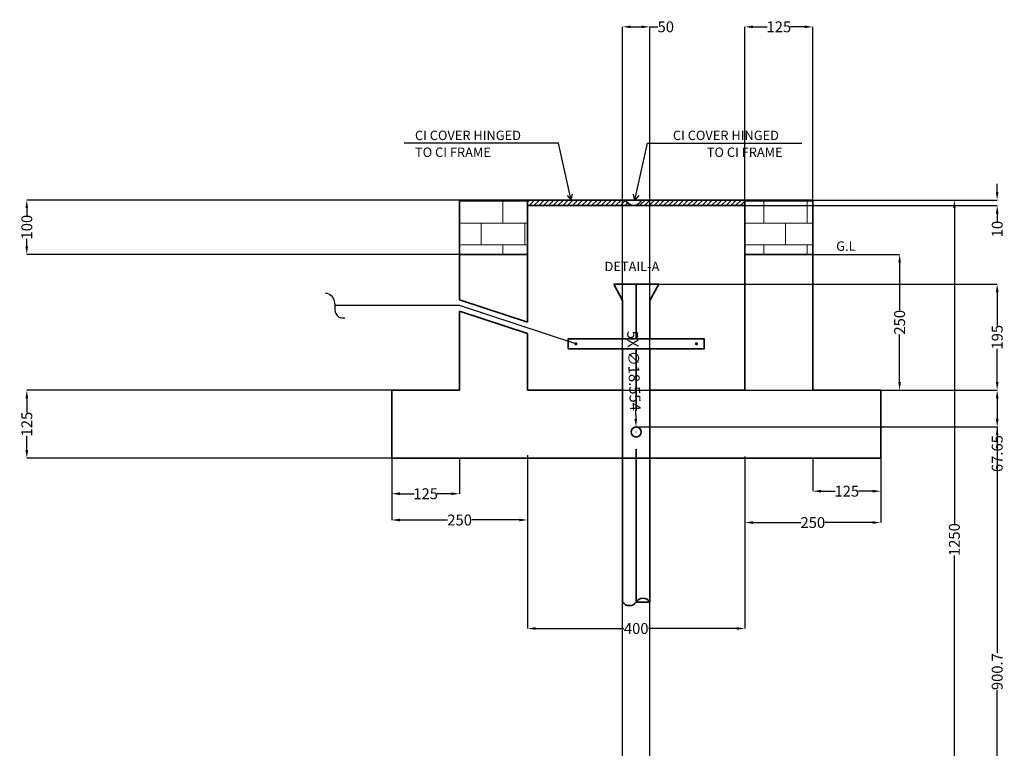
# Model space of a CAD drawing. Units: inches. Extents: x -129 to 2013, y -3652 to 814.
# Tile 5 of 5: x -129 to 1683, y -527 to 814. Entities that reach past the tile are written whole.
import ezdxf

# ---------------------------------------------------------------- set-up
doc = ezdxf.new("R2010")
doc.units = ezdxf.units.IN
doc.header["$MEASUREMENT"] = 0
for name, color, linetype, lineweight in [('A-ANNO-DIMS', 2, 'Continuous', 18), ('A-ANNO-TEXT', 7, 'Continuous', 25), ('A-DETL', 7, 'Continuous', 35), ('A-DETL-PATT', 8, 'Continuous', 13), ('E-GRND', 1, 'Continuous', 35)]:
    doc.layers.add(name, color=color, linetype=linetype, lineweight=lineweight)
doc.styles.get("Standard").update_dxf_attribs({"font": 'arial.ttf'})
doc.dimstyles.get("Standard").update_dxf_attribs({"dimtxt": 20, "dimasz": 15, "dimexe": 0.18, "dimexo": 0.0625, "dimgap": 0.09, "dimtad": 0, "dimdec": 0, "dimzin": 0, "dimdsep": 46, "dimtxsty": 'Standard', "dimcen": 0.09, "dimadec": 0, "dimazin": 0, "dimtfac": 1, "dimtdec": 0, "dimtofl": 0, "dimtmove": 0, "dimatfit": 3, "dimfxl": 1, "dimtolj": 1, "dimtzin": 0, "dimarcsym": 0})

# ---------------------------------------------------------------- blocks, each defined once
blk = doc.blocks.new('*D1')
at = {"layer": 'A-ANNO-DIMS', "color": 0, "lineweight": -2, "transparency": 16777216}
for p, q in [((1330.4, 382.4), (1490.1, 382.4)), ((1490, 367.4), (1490, 279.7)), ((1490, 147.4), (1490, 235)), ((1455.4, 132.4), (1490.1, 132.4))]:
    blk.add_line(p, q, dxfattribs=at)
at = {"layer": 'A-ANNO-DIMS', "color": 0, "transparency": 16777216}
for points in [[(1487.5, 367.4), (1492.5, 367.4), (1490, 382.4)], [(1487.5, 147.4), (1492.5, 147.4), (1490, 132.4)]]:
    blk.add_solid(points, dxfattribs=at)
at = {"layer": 'Defpoints', "color": 0, "transparency": 16777216}
for p in [(1330.3, 382.4), (1490, 382.4), (1455.3, 132.4)]:
    blk.add_point(p, dxfattribs=at)
at = {"layer": 'A-ANNO-DIMS', "color": 0, "transparency": 16777216, "insert": (1490, 257.4), "char_height": 20, "attachment_point": 5, "rotation": 90}
blk.add_mtext('\\A1;250', dxfattribs=at)
blk = doc.blocks.new('*D2')
at = {"layer": 'A-ANNO-DIMS', "color": 0, "lineweight": -2, "transparency": 16777216}
for p, q in [((1330.4, 482.4), (1591, 482.4)), ((1590.8, 467.4), (1590.8, -113.7)), ((1590.8, -752.6), (1590.8, -171.6)), ((1205.4, -767.6), (1591, -767.6))]:
    blk.add_line(p, q, dxfattribs=at)
at = {"layer": 'A-ANNO-DIMS', "color": 0, "transparency": 16777216}
for points in [[(1588.3, 467.4), (1593.3, 467.4), (1590.8, 482.4)], [(1588.3, -752.6), (1593.3, -752.6), (1590.8, -767.6)]]:
    blk.add_solid(points, dxfattribs=at)
at = {"layer": 'Defpoints', "color": 0, "transparency": 16777216}
for p in [(1330.3, 482.4), (1205.3, -767.6), (1590.8, -767.6)]:
    blk.add_point(p, dxfattribs=at)
at = {"layer": 'A-ANNO-DIMS', "color": 0, "transparency": 16777216, "insert": (1590.8, -142.6), "char_height": 20, "attachment_point": 5, "rotation": 90}
blk.add_mtext('\\A1;1250', dxfattribs=at)
blk = doc.blocks.new('*D4')
at = {"layer": 'A-ANNO-DIMS', "color": 0, "lineweight": -2, "transparency": 16777216}
for p, q in [((555.3, 7.3), (555.3, -58.3)), ((680.3, 7.3), (680.3, -58.3)), ((570.3, -58.2), (596.5, -58.2)), ((665.3, -58.2), (639.1, -58.2))]:
    blk.add_line(p, q, dxfattribs=at)
at = {"layer": 'A-ANNO-DIMS', "color": 0, "transparency": 16777216}
for points in [[(570.3, -55.7), (570.3, -60.7), (555.3, -58.2)], [(665.3, -55.7), (665.3, -60.7), (680.3, -58.2)]]:
    blk.add_solid(points, dxfattribs=at)
at = {"layer": 'Defpoints', "color": 0, "transparency": 16777216}
for p in [(555.3, 7.4), (680.3, 7.4), (680.3, -58.2)]:
    blk.add_point(p, dxfattribs=at)
at = {"layer": 'A-ANNO-DIMS', "color": 0, "transparency": 16777216, "insert": (617.8, -58.2), "char_height": 20, "attachment_point": 5}
blk.add_mtext('\\A1;125', dxfattribs=at)
blk = doc.blocks.new('*D5')
at = {"layer": 'A-ANNO-DIMS', "color": 0, "lineweight": -2, "transparency": 16777216}
for p, q in [((555.3, 7.3), (555.3, -106.7)), ((805.3, 12.7), (805.3, -106.7)), ((570.3, -106.5), (658, -106.5)), ((790.3, -106.5), (702.7, -106.5))]:
    blk.add_line(p, q, dxfattribs=at)
at = {"layer": 'A-ANNO-DIMS', "color": 0, "transparency": 16777216}
for points in [[(570.3, -104), (570.3, -109), (555.3, -106.5)], [(790.3, -104), (790.3, -109), (805.3, -106.5)]]:
    blk.add_solid(points, dxfattribs=at)
at = {"layer": 'Defpoints', "color": 0, "transparency": 16777216}
for p in [(555.3, 7.4), (805.3, 12.8), (805.3, -106.5)]:
    blk.add_point(p, dxfattribs=at)
at = {"layer": 'A-ANNO-DIMS', "color": 0, "transparency": 16777216, "insert": (680.3, -106.5), "char_height": 20, "attachment_point": 5}
blk.add_mtext('\\A1;250', dxfattribs=at)
blk = doc.blocks.new('*D6')
at = {"layer": 'A-ANNO-DIMS', "color": 0, "lineweight": -2, "transparency": 16777216}
for p, q in [((1330.3, 7.3), (1330.3, -53.6)), ((1455.3, 7.3), (1455.3, -53.6)), ((1345.3, -53.5), (1371.5, -53.5)), ((1440.3, -53.5), (1414.1, -53.5))]:
    blk.add_line(p, q, dxfattribs=at)
at = {"layer": 'A-ANNO-DIMS', "color": 0, "transparency": 16777216}
for points in [[(1345.3, -51), (1345.3, -56), (1330.3, -53.5)], [(1440.3, -51), (1440.3, -56), (1455.3, -53.5)]]:
    blk.add_solid(points, dxfattribs=at)
at = {"layer": 'Defpoints', "color": 0, "transparency": 16777216}
for p in [(1330.3, 7.4), (1455.3, 7.4), (1330.3, -53.5)]:
    blk.add_point(p, dxfattribs=at)
at = {"layer": 'A-ANNO-DIMS', "color": 0, "transparency": 16777216, "insert": (1392.8, -53.5), "char_height": 20, "attachment_point": 5}
blk.add_mtext('\\A1;125', dxfattribs=at)
blk = doc.blocks.new('*D7')
at = {"layer": 'A-ANNO-DIMS', "color": 0, "lineweight": -2, "transparency": 16777216}
for p, q in [((1455.3, 132.3), (1455.3, -111.4)), ((1205.3, 10.4), (1205.3, -111.4)), ((1220.3, -111.2), (1308, -111.2)), ((1440.3, -111.2), (1352.7, -111.2))]:
    blk.add_line(p, q, dxfattribs=at)
at = {"layer": 'A-ANNO-DIMS', "color": 0, "transparency": 16777216}
for points in [[(1220.3, -108.7), (1220.3, -113.7), (1205.3, -111.2)], [(1440.3, -108.7), (1440.3, -113.7), (1455.3, -111.2)]]:
    blk.add_solid(points, dxfattribs=at)
at = {"layer": 'Defpoints', "color": 0, "transparency": 16777216}
for p in [(1455.3, 132.4), (1205.3, 10.5), (1205.3, -111.2)]:
    blk.add_point(p, dxfattribs=at)
at = {"layer": 'A-ANNO-DIMS', "color": 0, "transparency": 16777216, "insert": (1330.3, -111.2), "char_height": 20, "attachment_point": 5}
blk.add_mtext('\\A1;250', dxfattribs=at)
blk = doc.blocks.new('*D8')
at = {"layer": 'A-ANNO-DIMS', "color": 0, "lineweight": -2, "transparency": 16777216}
for p, q in [((805.3, 7.3), (805.3, -306.4)), ((1205.3, 10.4), (1205.3, -306.4)), ((820.3, -306.2), (982.8, -306.2)), ((1190.3, -306.2), (1027.9, -306.2))]:
    blk.add_line(p, q, dxfattribs=at)
at = {"layer": 'A-ANNO-DIMS', "color": 0, "transparency": 16777216}
for points in [[(820.3, -303.7), (820.3, -308.7), (805.3, -306.2)], [(1190.3, -303.7), (1190.3, -308.7), (1205.3, -306.2)]]:
    blk.add_solid(points, dxfattribs=at)
at = {"layer": 'Defpoints', "color": 0, "transparency": 16777216}
for p in [(805.3, 7.4), (1205.3, 10.5), (805.3, -306.2)]:
    blk.add_point(p, dxfattribs=at)
at = {"layer": 'A-ANNO-DIMS', "color": 0, "transparency": 16777216, "insert": (1005.3, -306.2), "char_height": 20, "attachment_point": 5}
blk.add_mtext('\\A1;400', dxfattribs=at)
blk = doc.blocks.new('*D22')
at = {"layer": 'A-ANNO-DIMS', "color": 0, "lineweight": -2, "transparency": 16777216}
for p, q in [((555.3, 132.4), (-116.3, 132.4)), ((-116.2, 117.4), (-116.2, 91.2)), ((-116.2, 22.4), (-116.2, 48.5)), ((555.3, 7.4), (-116.3, 7.4))]:
    blk.add_line(p, q, dxfattribs=at)
at = {"layer": 'A-ANNO-DIMS', "color": 0, "transparency": 16777216}
for points in [[(-118.7, 117.4), (-113.7, 117.4), (-116.2, 132.4)], [(-118.7, 22.4), (-113.7, 22.4), (-116.2, 7.4)]]:
    blk.add_solid(points, dxfattribs=at)
at = {"layer": 'Defpoints', "color": 0, "transparency": 16777216}
for p in [(-116.2, 132.4), (555.3, 132.4), (555.3, 7.4)]:
    blk.add_point(p, dxfattribs=at)
at = {"layer": 'A-ANNO-DIMS', "color": 0, "transparency": 16777216, "insert": (-116.2, 69.9), "char_height": 20, "attachment_point": 5, "rotation": 90}
blk.add_mtext('\\A1;125', dxfattribs=at)
blk = doc.blocks.new('*D23')
at = {"layer": 'A-ANNO-DIMS', "color": 0, "lineweight": -2, "transparency": 16777216}
for p, q in [((680.3, 482.4), (-116.3, 482.4)), ((-116.2, 467.4), (-116.2, 453.6)), ((-116.2, 397.4), (-116.2, 411.2)), ((680.3, 382.4), (-116.3, 382.4))]:
    blk.add_line(p, q, dxfattribs=at)
at = {"layer": 'A-ANNO-DIMS', "color": 0, "transparency": 16777216}
for points in [[(-118.7, 467.4), (-113.7, 467.4), (-116.2, 482.4)], [(-118.7, 397.4), (-113.7, 397.4), (-116.2, 382.4)]]:
    blk.add_solid(points, dxfattribs=at)
at = {"layer": 'Defpoints', "color": 0, "transparency": 16777216}
for p in [(-116.2, 482.4), (680.3, 482.4), (680.3, 382.4)]:
    blk.add_point(p, dxfattribs=at)
at = {"layer": 'A-ANNO-DIMS', "color": 0, "transparency": 16777216, "insert": (-116.2, 432.4), "char_height": 20, "attachment_point": 5, "rotation": 90}
blk.add_mtext('\\A1;100', dxfattribs=at)
blk = doc.blocks.new('*D24')
at = {"layer": 'A-ANNO-DIMS', "color": 0, "lineweight": -2, "transparency": 16777216}
for p, q in [((1205.3, 482.4), (1205.3, 801.3)), ((1220.3, 801.1), (1246.5, 801.1)), ((1315.3, 801.1), (1289.1, 801.1)), ((1330.3, 482.4), (1330.3, 801.3))]:
    blk.add_line(p, q, dxfattribs=at)
at = {"layer": 'A-ANNO-DIMS', "color": 0, "transparency": 16777216}
for points in [[(1220.3, 803.6), (1220.3, 798.6), (1205.3, 801.1)], [(1315.3, 803.6), (1315.3, 798.6), (1330.3, 801.1)]]:
    blk.add_solid(points, dxfattribs=at)
at = {"layer": 'Defpoints', "color": 0, "transparency": 16777216}
for p in [(1330.3, 801.1), (1205.3, 482.4), (1330.3, 482.4)]:
    blk.add_point(p, dxfattribs=at)
at = {"layer": 'A-ANNO-DIMS', "color": 0, "transparency": 16777216, "insert": (1267.8, 801.1), "char_height": 20, "attachment_point": 5}
blk.add_mtext('\\A1;125', dxfattribs=at)
blk = doc.blocks.new('*D25')
at = {"layer": 'A-ANNO-DIMS', "color": 0, "lineweight": -2, "transparency": 16777216}
for p, q in [((1669.6, 497.4), (1669.6, 512.4)), ((805.4, 482.4), (1669.8, 482.4)), ((805.4, 472.4), (1669.8, 472.4)), ((1669.6, 457.4), (1669.6, 442.4))]:
    blk.add_line(p, q, dxfattribs=at)
at = {"layer": 'A-ANNO-DIMS', "color": 0, "transparency": 16777216}
for points in [[(1667.1, 497.4), (1672.1, 497.4), (1669.6, 482.4)], [(1667.1, 457.4), (1672.1, 457.4), (1669.6, 472.4)]]:
    blk.add_solid(points, dxfattribs=at)
at = {"layer": 'Defpoints', "color": 0, "transparency": 16777216}
for p in [(805.3, 482.4), (805.3, 472.4), (1669.6, 472.4)]:
    blk.add_point(p, dxfattribs=at)
at = {"layer": 'A-ANNO-DIMS', "color": 0, "transparency": 16777216, "insert": (1669.6, 428.9), "char_height": 20, "attachment_point": 5, "rotation": 90}
blk.add_mtext('\\A1;10', dxfattribs=at)
blk = doc.blocks.new('*D26')
at = {"layer": 'A-ANNO-DIMS', "color": 0, "lineweight": -2, "transparency": 16777216}
for p, q in [((980.3, -1867.6), (980.3, 801.3)), ((995.3, 801.1), (1015.3, 801.1)), ((1030.3, -1867.6), (1030.3, 801.3)), ((1030.3, 801.1), (1045.3, 801.1))]:
    blk.add_line(p, q, dxfattribs=at)
at = {"layer": 'A-ANNO-DIMS', "color": 0, "transparency": 16777216}
for points in [[(995.3, 803.6), (995.3, 798.6), (980.3, 801.1)], [(1015.3, 803.6), (1015.3, 798.6), (1030.3, 801.1)]]:
    blk.add_solid(points, dxfattribs=at)
at = {"layer": 'Defpoints', "color": 0, "transparency": 16777216}
for p in [(1030.3, 801.1), (980.3, -1867.6), (1030.3, -1867.6)]:
    blk.add_point(p, dxfattribs=at)
at = {"layer": 'A-ANNO-DIMS', "color": 0, "transparency": 16777216, "insert": (1059.7, 801.1), "char_height": 20, "attachment_point": 5}
blk.add_mtext('\\A1;50', dxfattribs=at)
blk = doc.blocks.new('*D27')
at = {"layer": 'A-ANNO-DIMS', "color": 0, "lineweight": -2, "transparency": 16777216}
for p, q in [((1046.7, 327.4), (1669.8, 327.4)), ((1669.6, 312.4), (1669.6, 251.2)), ((1669.6, 147.4), (1669.6, 208.5)), ((1205.4, 132.4), (1669.8, 132.4))]:
    blk.add_line(p, q, dxfattribs=at)
at = {"layer": 'A-ANNO-DIMS', "color": 0, "transparency": 16777216}
for points in [[(1667.1, 312.4), (1672.1, 312.4), (1669.6, 327.4)], [(1667.1, 147.4), (1672.1, 147.4), (1669.6, 132.4)]]:
    blk.add_solid(points, dxfattribs=at)
at = {"layer": 'Defpoints', "color": 0, "transparency": 16777216}
for p in [(1046.7, 327.4), (1205.3, 132.4), (1669.6, 132.4)]:
    blk.add_point(p, dxfattribs=at)
at = {"layer": 'A-ANNO-DIMS', "color": 0, "transparency": 16777216, "insert": (1669.6, 229.9), "char_height": 20, "attachment_point": 5, "rotation": 90}
blk.add_mtext('\\A1;195', dxfattribs=at)
blk = doc.blocks.new('*D28')
at = {"layer": 'A-ANNO-DIMS', "color": 0, "lineweight": -2, "transparency": 16777216}
for p, q in [((980.4, 132.4), (1669.8, 132.4)), ((1669.6, 117.4), (1669.6, 79.7)), ((1005.4, 64.7), (1669.8, 64.7)), ((1669.6, 64.7), (1669.6, 49.7))]:
    blk.add_line(p, q, dxfattribs=at)
at = {"layer": 'A-ANNO-DIMS', "color": 0, "transparency": 16777216}
for points in [[(1667.1, 117.4), (1672.1, 117.4), (1669.6, 132.4)], [(1667.1, 79.7), (1672.1, 79.7), (1669.6, 64.7)]]:
    blk.add_solid(points, dxfattribs=at)
at = {"layer": 'Defpoints', "color": 0, "transparency": 16777216}
for p in [(980.3, 132.4), (1005.3, 64.7), (1669.6, 64.7)]:
    blk.add_point(p, dxfattribs=at)
at = {"layer": 'A-ANNO-DIMS', "color": 0, "transparency": 16777216, "insert": (1669.6, 15.7), "char_height": 20, "attachment_point": 5, "rotation": 90}
blk.add_mtext('\\A1;67.65', dxfattribs=at)
blk = doc.blocks.new('*D29')
at = {"layer": 'A-ANNO-DIMS', "color": 0, "lineweight": -2, "transparency": 16777216}
for p, q in [((1005.4, 64.7), (1669.8, 64.7)), ((1669.6, 49.7), (1669.6, -351.8)), ((1669.6, -821), (1669.6, -419.5)), ((1005.4, -836), (1669.8, -836))]:
    blk.add_line(p, q, dxfattribs=at)
at = {"layer": 'A-ANNO-DIMS', "color": 0, "transparency": 16777216}
for points in [[(1667.1, 49.7), (1672.1, 49.7), (1669.6, 64.7)], [(1667.1, -821), (1672.1, -821), (1669.6, -836)]]:
    blk.add_solid(points, dxfattribs=at)
at = {"layer": 'Defpoints', "color": 0, "transparency": 16777216}
for p in [(1005.3, 64.7), (1005.3, -836), (1669.6, -836)]:
    blk.add_point(p, dxfattribs=at)
at = {"layer": 'A-ANNO-DIMS', "color": 0, "transparency": 16777216, "insert": (1669.6, -385.6), "char_height": 20, "attachment_point": 5, "rotation": 90}
blk.add_mtext('\\A1;900.7', dxfattribs=at)
blk = doc.blocks.new('*D34')
at = {"layer": 'A-ANNO-DIMS', "color": 0, "lineweight": -2, "transparency": 16777216}
for p, q in [((1003.9, 94.7), (1004.4, 79.7)), ((1005.2, 55.4), (1005.4, 55.4)), ((1005.3, 55.3), (1005.3, 55.5))]:
    blk.add_line(p, q, dxfattribs=at)
at = {"layer": 'A-ANNO-DIMS', "color": 0, "transparency": 16777216}
blk.add_solid([(1006.9, 79.8), (1001.9, 79.6), (1005, 64.7)], dxfattribs=at)
at = {"layer": 'Defpoints', "color": 0, "transparency": 16777216}
for p in [(1005, 64.7), (1005.7, 46.2)]:
    blk.add_point(p, dxfattribs=at)
at = {"layer": 'A-ANNO-DIMS', "color": 0, "transparency": 16777216, "insert": (1001.2, 168), "char_height": 20, "attachment_point": 5, "rotation": 272.0841}
blk.add_mtext('\\A1;5X ∅18.554', dxfattribs=at)

msp = doc.modelspace()

# ---------------------------------------------------------------- hatches: boundary and pattern name
at = {"layer": 'A-DETL-PATT'}
h = msp.add_hatch(dxfattribs=at)
h.set_pattern_fill('AR-B816', color=256, scale=5)
h.paths.add_polyline_path([(805.3299, 482.3603), (680.3299, 482.3603), (680.3299, 382.3603), (805.3299, 382.3603)])
h.paths.add_polyline_path([(1330.3299, 482.3603), (1205.3299, 482.3603), (1205.3299, 382.3603), (1330.3299, 382.3603)])
h = msp.add_hatch(dxfattribs=at)
h.set_pattern_fill('ANSI31', color=256, scale=50)
h.paths.add_polyline_path([(985.6513, 482.3603), (805.3299, 482.3603), (805.3299, 472.3603), (999.6786, 472.3603, -0.293221438)])
h.paths.add_polyline_path([(1205.3299, 482.3603), (1015.2644, 482.3603, -0.293221438), (1001.2372, 472.3603), (1205.3299, 472.3603)])

# ---------------------------------------------------------------- linework, layer by layer
at = {"layer": 'A-ANNO-TEXT'}
for points in [[(885.4212, 482.3603), (862.3427, 586.8686), (578.5573, 586.8686)], [(1002.9842, 482.3603), (1026.0627, 586.8686), (1309.8482, 586.8686)], [(878.2422, 490.9289), (885.4212, 482.3603), (888.3242, 493.1553)], [(1010.1632, 490.9289), (1002.9842, 482.3603), (1000.0813, 493.1553)], [(894.3429, 217.8056), (680.3299, 288.2653), (450.6375, 288.2653)]]:
    msp.add_lwpolyline(points, dxfattribs=at)
msp.add_open_spline([(433.1167, 311.7522), (437.1039, 310.5265), (447.7143, 307.2646), (451.4749, 289.5005), (450.2729, 275.0479), (458.3312, 265.1335), (465.1078, 265.27), (468.8937, 265.3463)], degree=3, knots=[0, 0, 0, 0, 11.88575847, 31.629827154, 46.748444814, 55.2513882, 66.015071682, 66.015071682, 66.015071682, 66.015071682], dxfattribs=at)
at = {"layer": 'A-DETL'}
for p, q in [((680.3299, 482.3603), (805.3299, 482.3603)), ((680.3299, 298.7933), (680.3299, 482.3603)), ((805.3299, 482.3603), (805.3299, 257.6395)), ((1330.3299, 482.3603), (805.3299, 482.3603)), ((805.3299, 257.6395), (805.3299, 482.3603)), ((1205.3299, 472.3603), (805.3299, 472.3603)), ((1205.3299, 482.3603), (1205.3299, 132.3603)), ((1205.3299, 132.3603), (1205.3299, 482.3603)), ((1330.3299, 132.3603), (1330.3299, 482.3603)), ((680.3299, 382.3603), (805.3299, 382.3603)), ((1330.3299, 382.3603), (1205.3299, 382.3603)), ((680.3299, 132.3603), (680.3299, 277.7373)), ((805.3299, 132.3603), (805.3299, 236.5834)), ((805.3299, 236.5834), (805.3299, 132.3603)), ((555.3299, 7.3603), (555.3299, 132.3603)), ((555.3299, 132.3603), (680.3299, 132.3603)), ((805.3299, 132.3603), (980.3299, 132.3603)), ((1030.3299, 132.3603), (1205.3299, 132.3603)), ((1455.3299, 132.3603), (1330.3299, 132.3603)), ((1455.3299, 7.3603), (1455.3299, 132.3603)), ((1455.3299, 7.3603), (555.3299, 7.3603))]:
    msp.add_line(p, q, dxfattribs=at)
msp.add_arc((1000.4579, 488.2916), 15.9504, 201.8304711, 338.1695289, dxfattribs=at)
at = {"layer": 'E-GRND'}
for p, q in [((1005.3299, 327.3549), (963.9747, 327.3549)), ((980.3299, 297.3549), (963.9747, 327.3549)), ((1005.3299, 327.3549), (1046.6851, 327.3549)), ((1005.3299, 227.1806), (1005.3299, 327.3549)), ((1046.6851, 327.3549), (1030.3299, 297.3549)), ((980.3299, 227.1806), (980.3299, 297.3549)), ((1030.3299, 227.1806), (1030.3299, 297.3549)), ((980.3299, -257.6028), (980.3299, 208.4306)), ((1005.3299, 94.7868), (1005.3299, 208.4306)), ((1030.3299, -257.6028), (1030.3299, 208.4306)), ((1005.3299, -257.6028), (1005.3299, 23.7551)), ((1030.3299, -257.8605), (1005.3299, -257.8605))]:
    msp.add_line(p, q, dxfattribs=at)
for points in [[(805.3299, 257.6395), (680.3299, 298.7933)], [(805.3299, 236.5834), (680.3299, 277.7373)]]:
    msp.add_lwpolyline(points, dxfattribs=at)
msp.add_lwpolyline([(880.3299, 208.4306), (1130.3299, 208.4306), (1130.3299, 227.1806), (880.3299, 227.1806)], close=True, dxfattribs=at)
at = {"layer": 'E-GRND', "const_width": 2.8735}
for points in [[(892.9062, 217.8056, 1), (895.7797, 217.8056, 1)], [(1117.7537, 217.8056, -1), (1114.8802, 217.8056, -1)]]:
    msp.add_lwpolyline(points, format="xyb", close=True, dxfattribs=at)
at = {"layer": 'E-GRND'}
msp.add_circle((1005.3299, 55.434), 9.277, dxfattribs=at)
for centre, radius, start, end in [((1017.8299, -264.8312), 14.3122, 29.1463796, 150.8536204), ((992.8299, -248.2393), 15.774, 217.5854091, 322.4145909)]:
    msp.add_arc(centre, radius, start, end, dxfattribs=at)

# ---------------------------------------------------------------- texts
at = {"layer": 'A-ANNO-TEXT'}
for s, height, p in [('CI COVER HINGED', 17.305551, (598.0639, 592.6904)), ('CI COVER HINGED', 17.305551, (1072.8181, 592.6904)), ('TO CI FRAME', 17.305551, (598.1704, 561.6597)), ('TO CI FRAME', 17.305551, (1135.1698, 561.6597)), ('G.L', 17.30555, (1373.3076, 388.8802)), ('DETAIL-A', 17.30555, (947.0009, 351.4317))]:
    msp.add_text(s, height=height, dxfattribs=at).set_placement(p)

# ---------------------------------------------------------------- dimensions: what is measured, and where the dimension line sits
at = {"layer": 'A-ANNO-DIMS'}
for base, p1, p2, override, picture, middle in [((1030.3299, 801.1186), (980.3299, -1867.6397), (1030.3299, -1867.6397), {"dimdec": 0, "dimlfac": 1, "dimrnd": 0, "dimzin": 0, "dimdsep": 46, "dimlunit": 2}, '*D26', (1059.7105, 801.1186)), ((1330.3299, 801.1186), (1205.3299, 482.3603), (1330.3299, 482.3603), {"dimdec": 0, "dimlfac": 1, "dimrnd": 0, "dimzin": 0, "dimdsep": 46, "dimlunit": 2}, '*D24', (1267.8299, 801.1186)), ((1205.3299, -111.1852), (1455.3299, 132.3603), (1205.3299, 10.4663), {"dimclrd": 0, "dimclre": 0, "dimclrt": 0}, '*D7', (1330.3299, -111.1852)), ((805.3299, -106.5375), (555.3299, 7.3603), (805.3299, 12.7901), {"dimclrd": 0, "dimclre": 0, "dimclrt": 0}, '*D5', (680.3299, -106.5375)), ((680.3299, -58.1694), (555.3299, 7.3603), (680.3299, 7.3603), {"dimclrd": 0, "dimclre": 0, "dimclrt": 0}, '*D4', (617.8299, -58.1694)), ((805.3299, -306.218), (1205.3299, 10.4663), (805.3299, 7.3603), {"dimclrd": 0, "dimclre": 0, "dimclrt": 0}, '*D8', (1005.3299, -306.218)), ((1330.3299, -53.4555), (1455.3299, 7.3603), (1330.3299, 7.3603), {"dimclrd": 0, "dimclre": 0, "dimclrt": 0}, '*D6', (1392.8299, -53.4555))]:
    dim = msp.add_linear_dim(base=base, p1=p1, p2=p2, dimstyle='Standard', override=override, dxfattribs=at)
    dim.commit()
    dim.dimension.update_dxf_attribs({"geometry": picture, "text_midpoint": middle})
for base, p1, p2, override, picture, middle in [((1669.5799, 472.3603), (805.3299, 482.3603), (805.3299, 472.3603), {"dimdec": 0, "dimlfac": 1, "dimrnd": 0, "dimzin": 0, "dimdsep": 46, "dimlunit": 2}, '*D25', (1669.5799, 428.921)), ((-116.1573, 482.3603), (680.3299, 382.3603), (680.3299, 482.3603), {"dimdec": 0, "dimlfac": 1, "dimrnd": 0, "dimzin": 0, "dimdsep": 46, "dimlunit": 2}, '*D23', (-116.1573, 432.3603)), ((1590.798, -767.6397), (1330.3299, 482.3603), (1205.3299, -767.6397), {"dimclrd": 0, "dimclre": 0, "dimclrt": 0}, '*D2', (1590.798, -142.6397)), ((1489.9699, 382.3603), (1455.3299, 132.3603), (1330.3299, 382.3603), {"dimclrd": 0, "dimclre": 0, "dimclrt": 0}, '*D1', (1489.9699, 257.3603)), ((1669.5799, 132.3603), (1046.6851, 327.3549), (1205.3299, 132.3603), {"dimdec": 0, "dimlfac": 1, "dimrnd": 0, "dimzin": 0, "dimdsep": 46, "dimlunit": 2}, '*D27', (1669.5799, 229.8576)), ((-116.1573, 132.3603), (555.3299, 7.3603), (555.3299, 132.3603), {"dimdec": 0, "dimlfac": 1, "dimrnd": 0, "dimzin": 0, "dimdsep": 46, "dimlunit": 2}, '*D22', (-116.1573, 69.8603)), ((1669.5799, 64.711), (980.3299, 132.3603), (1005.3299, 64.711), {"dimdec": 2, "dimlfac": 1, "dimrnd": 0, "dimzin": 0, "dimdsep": 46, "dimlunit": 2}, '*D28', (1669.5799, 15.7465)), ((1669.5799, -835.9565), (1005.3299, 64.711), (1005.3299, -835.9565), {"dimdec": 1, "dimlfac": 1, "dimrnd": 0, "dimzin": 0, "dimdsep": 46, "dimlunit": 2}, '*D29', (1669.5799, -385.6228))]:
    dim = msp.add_linear_dim(base=base, p1=p1, p2=p2, angle=90, dimstyle='Standard', override=override, dxfattribs=at)
    dim.commit()
    dim.dimension.update_dxf_attribs({"geometry": picture, "text_midpoint": middle})
dim = msp.add_diameter_dim_2p(p1=(1005.6673, 46.1631), p2=(1004.9925, 64.7048), text='5X <>', dimstyle='Standard', override={"dimdec": 3, "dimlfac": 1, "dimrnd": 0, "dimzin": 0, "dimdsep": 46, "dimlunit": 2}, dxfattribs=at)
dim.commit()
dim.dimension.update_dxf_attribs({"geometry": '*D34', "text_midpoint": (1001.2323, 168.0347)})

doc.saveas('drawing.dxf')
